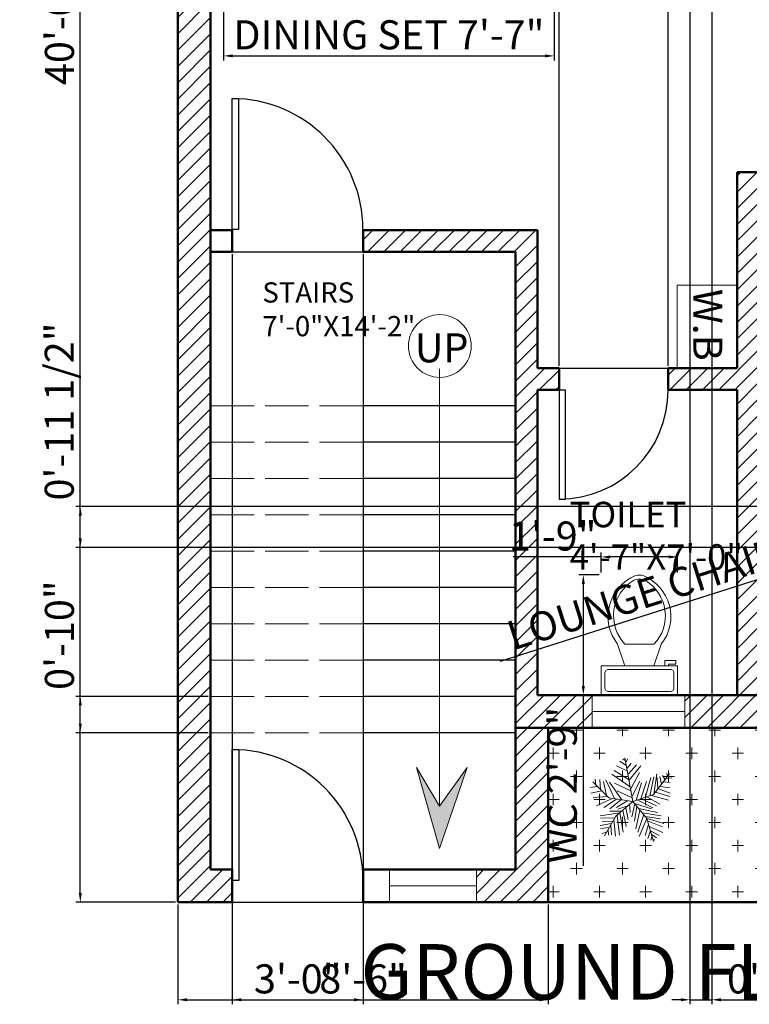
# Model space of a CAD drawing. Units: inches. Extents: x 1188 to 1681, y 1982 to 2608.
# Tile 1 of 4: x 1188 to 1389, y 1988 to 2259. Entities that reach past the tile are written whole.
import ezdxf

# ---------------------------------------------------------------- set-up
doc = ezdxf.new("R2010")
doc.units = ezdxf.units.IN
doc.linetypes.add('ACAD_ISO02W100', pattern=[15, 12, -3])
for name, color, linetype, lineweight in [('A-ANNO-DIMS', 2, 'Continuous', 18), ('A-ANNO-SYMB', 7, 'Continuous', 18), ('A-ANNO-TEXT', 7, 'Continuous', 25), ('A-AREA-IDEN', 7, 'Continuous', 18), ('A-DOOR', 4, 'Continuous', 25), ('A-FLOR-FIXT', 9, 'Continuous', 18), ('A-FLOR-STRS', 7, 'Continuous', 25), ('A-FLOR-STRS-OVHD', 8, 'ACAD_ISO02W100', 18), ('A-GLAZ', 4, 'Continuous', 20), ('A-WALL', 7, 'Continuous', 50), ('A-WALL-PATT', 8, 'Continuous', 13)]:
    doc.layers.add(name, color=color, linetype=linetype, lineweight=lineweight)
doc.layers.add('L-PLNT', color=116, linetype='Continuous', lineweight=18, true_color=0x136734)
doc.layers.add('L-PLNT-PATT', color=116, linetype='Continuous', lineweight=13, true_color=0x136734)
doc.styles.get("Standard").update_dxf_attribs({"font": 'arial.ttf'})
doc.dimstyles.new('ISO-25', dxfattribs={"dimtxt": 8, "dimasz": 2.5, "dimexe": 1.25, "dimexo": 0.625, "dimtad": 1, "dimdec": 1, "dimlunit": 4, "dimtxsty": 'Standard', "dimcen": 2.5, "dimadec": 0, "dimazin": 0, "dimtfac": 1, "dimtdec": 1, "dimtmove": 0, "dimatfit": 3, "dimfxl": 1, "dimarcsym": 0})

# ---------------------------------------------------------------- blocks, each defined once
blk = doc.blocks.new('*U2')
for p, q in [((0, 0), (0, -6)), ((36, 0), (36, -6))]:
    blk.add_line(p, q)
blk.add_lwpolyline([(0, 0), (0, 36), (1.75, 36), (1.75, 0)], close=True)
blk.add_arc((0, 0), 36, 0, 90)
blk = doc.blocks.new('*U3')
for p, q in [((0, 0), (0, 6)), ((30, 0), (30, 6))]:
    blk.add_line(p, q)
blk.add_lwpolyline([(0, 0), (0, -30), (1.75, -30), (1.75, 0)], close=True)
blk.add_arc((0, 0), 30, 270, 0)
blk = doc.blocks.new('Toilet - top')
for p, q in [((9.5, -6), (9.5, -2)), ((-8, -8.5), (-8, -8)), ((-7, -8), (-7, -9.5)), ((-4, -8), (-6, -14)), ((4, -8), (6, -14)), ((-10, -8.5), (-8, -8.5)), ((-10, -9.5), (-10, -8.5)), ((-7, -9.5), (-10, -9.5)), ((4, -14), (-4, -14))]:
    blk.add_line(p, q)
blk.add_lwpolyline([(10.5, -8), (10.5, 0), (-10.5, 0), (-10.5, -8)], close=True)
for points in [[(-9.5, -2), (-9.5, -6)], [(8.5, -1), (-8.5, -1)], [(-8.5, -7), (8.5, -7)]]:
    blk.add_lwpolyline(points)
for centre, radius, start, end in [((-8.62, -1.88), 0.884, 81.8699, 188.1301), ((8.62, -1.88), 0.884, 351.8699, 98.1301), ((-8.62, -6.12), 0.884, 171.8699, 278.1301), ((8.62, -6.12), 0.884, 261.8699, 8.1301), ((3.52, -21.58), 12.17, 141.4691, 247.9714), ((4.2, -21.82), 11.33, 136.3677, 238.9468), ((-3.52, -21.58), 12.17, 292.0284, 38.5307), ((-4.2, -21.82), 11.33, 301.053, 43.6321), ((0, -27.88), 4, 245.7318, 294.2682), ((0, -29), 4, 254.8605, 285.1395)]:
    blk.add_arc(centre, radius, start, end)
blk = doc.blocks.new('*U12')
for p, q in [((-8.737, 47.138), (-17.069, 52.711)), ((-10.186, 53.64), (-13.084, 55.962)), ((0, 0), (-10.5, 57)), ((-9.099, 51.782), (-6.563, 55.962)), ((-5.114, 28.097), (-24.676, 40.636)), ((-7.288, 39.707), (-21.778, 46.673)), ((-7.65, 43.423), (-2.578, 49.46)), ((-5.839, 35.992), (4.667, 48.067)), ((-5.114, 27.632), (10.463, 46.673)), ((-48.585, 21.131), (-49.309, 29.026)), ((-43.513, 28.561), (-42.427, 15.558)), ((-38.442, 26.239), (-34.819, 7.663)), ((-35.544, 28.097), (-24.314, 3.947)), ((-3.665, 19.273), (-27.574, 35.527)), ((-2.941, 16.486), (8.652, 37.85)), ((-1.129, 6.734), (9.014, 26.704)), ((10.101, 3.483), (17.708, 26.239)), ((16.259, 5.805), (23.142, 31.348)), ((22.055, 7.198), (27.489, 32.277)), ((27, 9), (48, 36)), ((27.127, 9.056), (31.112, 35.992)), ((31.836, 30.883), (32.561, 16.486)), ((35.096, 32.741), (37.27, 22.524)), ((38.719, 34.134), (41.979, 28.561)), ((43.791, 29.954), (51.036, 30.883)), ((44.153, 36.456), (45.239, 32.741)), ((-47.498, 19.737), (-55.83, 18.344)), ((-40.615, 13.7), (-55.105, 10.913)), ((-31.5, 4.5), (-52.5, 25.5)), ((-14.533, 2.09), (-30.834, 25.31)), ((-24.314, 23.917), (-2.941, 13.7)), ((-20.691, 13.7), (-1.129, 4.876)), ((3.942, 1.625), (11.187, 24.381)), ((33.285, 16.486), (48.862, 10.913)), ((36.183, 19.737), (48.137, 17.88)), ((40.53, 25.775), (48.862, 24.846)), ((-33.37, 6.269), (-52.207, 5.34)), ((-28.299, 3.483), (-47.86, -5.805)), ((-21.416, 3.018), (-38.079, -8.128)), ((0, 0), (-31.5, 4.5)), ((-15.982, 2.09), (-30.11, -9.521)), ((0, 0), (-22.5, -19.5)), ((-6.563, 1.161), (-21.416, -8.128)), ((0, 0), (27, 9)), ((0, 0), (18, -22.5)), ((6.478, 1.625), (26.04, -8.592)), ((11.187, 3.483), (30.749, -5.805)), ((18.07, 5.805), (35.096, -3.483)), ((24.229, 7.663), (46.688, 1.625)), ((29.662, 12.307), (48.137, 6.269)), ((-15.257, -12.772), (-30.11, -12.772)), ((-6.563, -5.805), (-19.967, -9.985)), ((-13.446, -11.378), (-8.737, -32.741)), ((-9.461, -8.592), (-6.201, -23.453)), ((-4.752, -3.483), (-3.665, -14.629)), ((2.493, -3.019), (-1.491, -20.202)), ((1.769, -2.555), (24.229, -9.521)), ((5.029, -6.27), (2.131, -25.775)), ((9.014, -11.378), (3.58, -35.992)), ((7.565, -9.056), (32.198, -14.629)), ((-17.431, -15.094), (-42.789, -18.809)), ((-24.314, -21.596), (-42.427, -22.06)), ((-26.849, -26.24), (-40.253, -25.775)), ((-22.5, -19.5), (-37.5, -45)), ((-25.038, -23.918), (-22.865, -45.281)), ((-20.691, -18.345), (-17.793, -44.352)), ((-17.069, -15.094), (-12.721, -40.172)), ((14.085, -16.951), (6.478, -40.172)), ((18.07, -22.524), (8.289, -45.745)), ((12.274, -15.094), (36.907, -18.809)), ((16.259, -19.738), (36.183, -22.989)), ((18, -22.5), (27, -52.5)), ((18.433, -22.524), (40.53, -29.026)), ((19.157, -25.311), (38.719, -33.206)), ((-28.299, -29.026), (-42.789, -31.348)), ((-30.834, -34.135), (-42.427, -35.528)), ((-32.646, -36.921), (-31.921, -44.352)), ((-29.023, -30.884), (-27.936, -43.887)), ((20.244, -30.419), (15.897, -44.816)), ((22.78, -37.85), (19.519, -48.532)), ((21.331, -32.741), (39.081, -40.636)), ((22.78, -38.314), (34.372, -44.816)), ((-34.457, -39.708), (-40.978, -42.494)), ((24.591, -45.745), (23.142, -50.854)), ((24.591, -43.423), (30.749, -47.603)), ((26.764, -49.925), (28.213, -50.854))]:
    blk.add_line(p, q)
blk = doc.blocks.new('*D30')
at = {"layer": 'A-ANNO-DIMS', "color": 0, "lineweight": -2, "transparency": 16777216}
for p, q in [((1498.32, 2135.79), (1496.92, 2140.18)), ((1494.92, 2138.23), (1474.36, 2131.69)), ((1471.98, 2130.93), (1320.5, 2082.67)), ((1473, 2127.73), (1471.6, 2132.12))]:
    blk.add_line(p, q, dxfattribs=at)
at = {"layer": 'A-ANNO-DIMS', "color": 0, "transparency": 16777216}
for points in [[(1494.79, 2138.63), (1495.04, 2137.84), (1497.3, 2138.99)], [(1474.24, 2132.08), (1474.49, 2131.29), (1471.98, 2130.93)]]:
    blk.add_solid(points, dxfattribs=at)
at = {"layer": 'Defpoints', "color": 0, "transparency": 16777216}
for p in [(1498.51, 2135.2), (1471.98, 2130.93), (1473.19, 2127.13)]:
    blk.add_point(p, dxfattribs=at)
at = {"layer": 'A-ANNO-DIMS', "color": 0, "transparency": 16777216, "insert": (1393.6, 2110.96), "char_height": 8, "attachment_point": 5, "rotation": 17.6695}
blk.add_mtext('LOUNGE CHAIR 2\'-2 1/2" TYP.', dxfattribs=at)
blk = doc.blocks.new('*D32')
at = {"layer": 'A-ANNO-DIMS', "color": 0, "lineweight": -2, "transparency": 16777216}
for p, q in [((1419.52, 2095.98), (1419.52, 2243.74)), ((1418.76, 2095.98), (1420.77, 2095.98)), ((1419.52, 2089.2), (1419.52, 2093.48)), ((1418.76, 2086.7), (1420.77, 2086.7))]:
    blk.add_line(p, q, dxfattribs=at)
at = {"layer": 'A-ANNO-DIMS', "color": 0, "transparency": 16777216}
for points in [[(1419.11, 2093.48), (1419.94, 2093.48), (1419.52, 2095.98)], [(1419.11, 2089.2), (1419.94, 2089.2), (1419.52, 2086.7)]]:
    blk.add_solid(points, dxfattribs=at)
at = {"layer": 'Defpoints', "color": 0, "transparency": 16777216}
for p in [(1418.13, 2095.98), (1419.52, 2095.98), (1418.13, 2086.7)]:
    blk.add_point(p, dxfattribs=at)
at = {"layer": 'A-ANNO-DIMS', "color": 0, "transparency": 16777216, "insert": (1414.76, 2171.11), "char_height": 8, "attachment_point": 5, "rotation": 90}
blk.add_mtext('RADIAL LAMP 0\'-9 1/2" TYP.', dxfattribs=at)
blk = doc.blocks.new('*D38')
at = {"layer": 'A-ANNO-DIMS', "color": 0, "lineweight": -2, "transparency": 16777216}
for p, q in [((1244.32, 2262.4), (1244.32, 2248.12)), ((1335.32, 2262.4), (1335.32, 2248.12)), ((1246.82, 2249.37), (1332.82, 2249.37))]:
    blk.add_line(p, q, dxfattribs=at)
at = {"layer": 'A-ANNO-DIMS', "color": 0, "transparency": 16777216}
for points in [[(1246.82, 2249.79), (1246.82, 2248.96), (1244.32, 2249.37)], [(1332.82, 2249.79), (1332.82, 2248.96), (1335.32, 2249.37)]]:
    blk.add_solid(points, dxfattribs=at)
at = {"layer": 'Defpoints', "color": 0, "transparency": 16777216}
for p in [(1244.32, 2263.02), (1335.32, 2263.02), (1335.32, 2249.37)]:
    blk.add_point(p, dxfattribs=at)
at = {"layer": 'A-ANNO-DIMS', "color": 0, "transparency": 16777216, "insert": (1289.82, 2254.14), "char_height": 8, "attachment_point": 5}
blk.add_mtext('DINING SET 7\'-7"', dxfattribs=at)
blk = doc.blocks.new('*D42')
at = {"layer": 'A-ANNO-DIMS', "color": 0, "lineweight": -2, "transparency": 16777216}
for p, q in [((1347.68, 2106.5), (1342.1, 2106.5)), ((1343.35, 2104), (1343.35, 2075.96)), ((1347.68, 2073.46), (1342.1, 2073.46)), ((1343.35, 2073.46), (1343.35, 2026.39))]:
    blk.add_line(p, q, dxfattribs=at)
at = {"layer": 'A-ANNO-DIMS', "color": 0, "transparency": 16777216}
for points in [[(1342.93, 2104), (1343.77, 2104), (1343.35, 2106.5)], [(1342.93, 2075.96), (1343.77, 2075.96), (1343.35, 2073.46)]]:
    blk.add_solid(points, dxfattribs=at)
at = {"layer": 'Defpoints', "color": 0, "transparency": 16777216}
for p in [(1348.31, 2106.5), (1343.35, 2073.46), (1348.31, 2073.46)]:
    blk.add_point(p, dxfattribs=at)
at = {"layer": 'A-ANNO-DIMS', "color": 0, "transparency": 16777216, "insert": (1338.59, 2048.67), "char_height": 8, "attachment_point": 5, "rotation": 90}
blk.add_mtext('WC 2\'-9"', dxfattribs=at)
blk = doc.blocks.new('*D43')
at = {"layer": 'A-ANNO-DIMS', "color": 0, "lineweight": -2, "transparency": 16777216}
for p, q in [((1348.31, 2111.46), (1324.04, 2111.46)), ((1348.31, 2107.13), (1348.31, 2112.71)), ((1366.81, 2111.46), (1350.81, 2111.46)), ((1369.31, 2107.13), (1369.31, 2112.71))]:
    blk.add_line(p, q, dxfattribs=at)
at = {"layer": 'A-ANNO-DIMS', "color": 0, "transparency": 16777216}
for points in [[(1350.81, 2111.88), (1350.81, 2111.04), (1348.31, 2111.46)], [(1366.81, 2111.88), (1366.81, 2111.04), (1369.31, 2111.46)]]:
    blk.add_solid(points, dxfattribs=at)
at = {"layer": 'Defpoints', "color": 0, "transparency": 16777216}
for p in [(1348.31, 2111.46), (1348.31, 2106.5), (1369.31, 2106.5)]:
    blk.add_point(p, dxfattribs=at)
at = {"layer": 'A-ANNO-DIMS', "color": 0, "transparency": 16777216, "insert": (1334.93, 2116.17), "char_height": 8, "attachment_point": 5}
blk.add_mtext('1\'-9"', dxfattribs=at)
blk = doc.blocks.new('*D44')
at = {"layer": 'A-ANNO-DIMS', "color": 0, "lineweight": -2, "transparency": 16777216}
for p, q in [((1231.09, 2496.41), (1203.62, 2496.41)), ((1204.87, 2018.91), (1204.87, 2493.91)), ((1231.09, 2016.41), (1203.62, 2016.41))]:
    blk.add_line(p, q, dxfattribs=at)
at = {"layer": 'A-ANNO-DIMS', "color": 0, "transparency": 16777216}
for points in [[(1204.45, 2493.91), (1205.28, 2493.91), (1204.87, 2496.41)], [(1204.45, 2018.91), (1205.28, 2018.91), (1204.87, 2016.41)]]:
    blk.add_solid(points, dxfattribs=at)
at = {"layer": 'Defpoints', "color": 0, "transparency": 16777216}
for p in [(1204.87, 2496.41), (1231.72, 2496.41), (1231.72, 2016.41)]:
    blk.add_point(p, dxfattribs=at)
at = {"layer": 'A-ANNO-DIMS', "color": 0, "transparency": 16777216, "insert": (1200.16, 2256.41), "char_height": 8, "attachment_point": 5, "rotation": 90}
blk.add_mtext('40\'-0"', dxfattribs=at)
blk = doc.blocks.new('*D45')
at = {"layer": 'A-ANNO-DIMS', "color": 0, "lineweight": -2, "transparency": 16777216}
for p, q in [((1246.72, 2015.79), (1246.72, 1988.31)), ((1282.72, 2015.79), (1282.72, 1988.31)), ((1249.22, 1989.56), (1280.22, 1989.56))]:
    blk.add_line(p, q, dxfattribs=at)
at = {"layer": 'A-ANNO-DIMS', "color": 0, "transparency": 16777216}
for points in [[(1249.22, 1989.98), (1249.22, 1989.15), (1246.72, 1989.56)], [(1280.22, 1989.98), (1280.22, 1989.15), (1282.72, 1989.56)]]:
    blk.add_solid(points, dxfattribs=at)
at = {"layer": 'Defpoints', "color": 0, "transparency": 16777216}
for p in [(1246.72, 2016.41), (1282.72, 2016.41), (1282.72, 1989.56)]:
    blk.add_point(p, dxfattribs=at)
at = {"layer": 'A-ANNO-DIMS', "color": 0, "transparency": 16777216, "insert": (1264.72, 1994.28), "char_height": 8, "attachment_point": 5}
blk.add_mtext('3\'-0"', dxfattribs=at)
blk = doc.blocks.new('*D46')
at = {"layer": 'A-ANNO-DIMS', "color": 0, "lineweight": -2, "transparency": 16777216}
for p, q in [((1204.87, 2073.07), (1204.87, 2104.3)), ((1240.09, 2073.07), (1203.62, 2073.07)), ((1204.87, 2065.57), (1204.87, 2070.57)), ((1240.09, 2063.07), (1203.62, 2063.07))]:
    blk.add_line(p, q, dxfattribs=at)
at = {"layer": 'A-ANNO-DIMS', "color": 0, "transparency": 16777216}
for points in [[(1204.45, 2070.57), (1205.28, 2070.57), (1204.87, 2073.07)], [(1204.45, 2065.57), (1205.28, 2065.57), (1204.87, 2063.07)]]:
    blk.add_solid(points, dxfattribs=at)
at = {"layer": 'Defpoints', "color": 0, "transparency": 16777216}
for p in [(1204.87, 2073.07), (1240.72, 2073.07), (1240.72, 2063.07)]:
    blk.add_point(p, dxfattribs=at)
at = {"layer": 'A-ANNO-DIMS', "color": 0, "transparency": 16777216, "insert": (1200.16, 2089.93), "char_height": 8, "attachment_point": 5, "rotation": 90}
blk.add_mtext('0\'-10"', dxfattribs=at)
blk = doc.blocks.new('*D47')
at = {"layer": 'A-ANNO-DIMS', "color": 0, "lineweight": -2, "transparency": 16777216}
for p, q in [((1336.72, 2164.04), (1336.72, 2524.51)), ((1339.22, 2523.26), (1364.22, 2523.26)), ((1366.72, 2164.04), (1366.72, 2524.51))]:
    blk.add_line(p, q, dxfattribs=at)
at = {"layer": 'A-ANNO-DIMS', "color": 0, "transparency": 16777216}
for points in [[(1339.22, 2523.68), (1339.22, 2522.85), (1336.72, 2523.26)], [(1364.22, 2523.68), (1364.22, 2522.85), (1366.72, 2523.26)]]:
    blk.add_solid(points, dxfattribs=at)
at = {"layer": 'Defpoints', "color": 0, "transparency": 16777216}
for p in [(1366.72, 2523.26), (1336.72, 2163.41), (1366.72, 2163.41)]:
    blk.add_point(p, dxfattribs=at)
at = {"layer": 'A-ANNO-DIMS', "color": 0, "transparency": 16777216, "insert": (1351.72, 2527.97), "char_height": 8, "attachment_point": 5}
blk.add_mtext('2\'-6"', dxfattribs=at)
blk = doc.blocks.new('*D49')
at = {"layer": 'A-ANNO-DIMS', "color": 0, "lineweight": -2, "transparency": 16777216}
for p, q in [((1231.72, 2015.79), (1231.72, 1988.31)), ((1333.72, 2015.79), (1333.72, 1988.31)), ((1234.22, 1989.56), (1331.22, 1989.56))]:
    blk.add_line(p, q, dxfattribs=at)
at = {"layer": 'A-ANNO-DIMS', "color": 0, "transparency": 16777216}
for points in [[(1234.22, 1989.98), (1234.22, 1989.15), (1231.72, 1989.56)], [(1331.22, 1989.98), (1331.22, 1989.15), (1333.72, 1989.56)]]:
    blk.add_solid(points, dxfattribs=at)
at = {"layer": 'Defpoints', "color": 0, "transparency": 16777216}
for p in [(1231.72, 2016.41), (1333.72, 2016.41), (1333.72, 1989.56)]:
    blk.add_point(p, dxfattribs=at)
at = {"layer": 'A-ANNO-DIMS', "color": 0, "transparency": 16777216, "insert": (1282.72, 1994.27), "char_height": 8, "attachment_point": 5}
blk.add_mtext('8\'-6"', dxfattribs=at)
blk = doc.blocks.new('*D50')
at = {"layer": 'A-ANNO-DIMS', "color": 0, "lineweight": -2, "transparency": 16777216}
for p, q in [((1372.72, 2342.79), (1372.72, 1988.31)), ((1378.72, 2336.79), (1378.72, 1988.31)), ((1370.22, 1989.56), (1367.72, 1989.56)), ((1372.72, 1989.56), (1378.72, 1989.56)), ((1381.22, 1989.56), (1406.23, 1989.56))]:
    blk.add_line(p, q, dxfattribs=at)
at = {"layer": 'A-ANNO-DIMS', "color": 0, "transparency": 16777216}
for points in [[(1370.22, 1989.98), (1370.22, 1989.15), (1372.72, 1989.56)], [(1381.22, 1989.98), (1381.22, 1989.15), (1378.72, 1989.56)]]:
    blk.add_solid(points, dxfattribs=at)
at = {"layer": 'Defpoints', "color": 0, "transparency": 16777216}
for p in [(1372.72, 2343.41), (1378.72, 2337.41), (1378.72, 1989.56)]:
    blk.add_point(p, dxfattribs=at)
at = {"layer": 'A-ANNO-DIMS', "color": 0, "transparency": 16777216, "insert": (1394.97, 1994.27), "char_height": 8, "attachment_point": 5}
blk.add_mtext('0\'-6"', dxfattribs=at)
blk = doc.blocks.new('*D56')
at = {"layer": 'A-ANNO-DIMS', "color": 0, "lineweight": -2, "transparency": 16777216}
for p, q in [((1246.72, 2194.79), (1246.72, 1988.31)), ((1282.72, 2194.79), (1282.72, 1988.31)), ((1249.22, 1989.56), (1280.22, 1989.56))]:
    blk.add_line(p, q, dxfattribs=at)
at = {"layer": 'A-ANNO-DIMS', "color": 0, "transparency": 16777216}
for points in [[(1249.22, 1989.98), (1249.22, 1989.15), (1246.72, 1989.56)], [(1280.22, 1989.98), (1280.22, 1989.15), (1282.72, 1989.56)]]:
    blk.add_solid(points, dxfattribs=at)
at = {"layer": 'Defpoints', "color": 0, "transparency": 16777216}
for p in [(1246.72, 2195.41), (1282.72, 2195.41), (1282.72, 1989.56)]:
    blk.add_point(p, dxfattribs=at)
at = {"layer": 'A-ANNO-DIMS', "color": 0, "transparency": 16777216, "insert": (1264.72, 1994.28), "char_height": 8, "attachment_point": 5}
blk.add_mtext('3\'-0"', dxfattribs=at)
blk = doc.blocks.new('*D58')
at = {"layer": 'A-ANNO-DIMS', "color": 0, "lineweight": -2, "transparency": 16777216}
for p, q in [((1204.87, 2125.31), (1204.87, 2175.18)), ((1439.4, 2125.31), (1203.62, 2125.31)), ((1204.87, 2116.54), (1204.87, 2122.81)), ((1439.4, 2114.04), (1203.62, 2114.04))]:
    blk.add_line(p, q, dxfattribs=at)
at = {"layer": 'A-ANNO-DIMS', "color": 0, "transparency": 16777216}
for points in [[(1204.45, 2122.81), (1205.28, 2122.81), (1204.87, 2125.31)], [(1204.45, 2116.54), (1205.28, 2116.54), (1204.87, 2114.04)]]:
    blk.add_solid(points, dxfattribs=at)
at = {"layer": 'Defpoints', "color": 0, "transparency": 16777216}
for p in [(1204.87, 2125.31), (1440.02, 2125.31), (1440.02, 2114.04)]:
    blk.add_point(p, dxfattribs=at)
at = {"layer": 'A-ANNO-DIMS', "color": 0, "transparency": 16777216, "insert": (1200.11, 2151.49), "char_height": 8, "attachment_point": 5, "rotation": 90}
blk.add_mtext('0\'-11 1/2"', dxfattribs=at)

msp = doc.modelspace()

# ---------------------------------------------------------------- hatches: boundary and pattern name
at = {"layer": 'A-ANNO-SYMB', "transparency": 33554564}
h = msp.add_hatch(color=256, dxfattribs=at)
h.dxf.hatch_style = 1
h.paths.add_polyline_path([(1311.34, 2053.46), (1303.72, 2042.82), (1297.4, 2053.46), (1303.72, 2031.22)])
at = {"layer": 'A-WALL-PATT', "transparency": 33554559}
h = msp.add_hatch(dxfattribs=at)
h.set_pattern_fill('ANSI31', color=256)
h.paths.add_polyline_path([(1390.99, 2496.41), (1231.72, 2496.41), (1231.72, 2452.82), (1240.72, 2452.82), (1240.72, 2487.41), (1390.99, 2487.41)])
h.paths.add_polyline_path([(1469.3, 2496.41), (1426.99, 2496.41), (1426.99, 2491.91), (1426.99, 2487.41), (1469.3, 2487.41)])
h.paths.add_polyline_path([(1378.72, 2487.41), (1372.72, 2487.41), (1372.72, 2404.84), (1372.72, 2343.41), (1367.48, 2343.41), (1367.48, 2337.41), (1378.72, 2337.41), (1378.72, 2391.41), (1387.67, 2391.41), (1387.67, 2397.41), (1378.72, 2397.41)])
h.paths.add_polyline_path([(1438.72, 2487.41), (1432.72, 2487.41), (1432.72, 2397.41), (1420.72, 2397.41), (1420.72, 2391.41), (1432.72, 2391.41), (1432.72, 2385.41), (1438.72, 2385.41)])
h.paths.add_polyline_path([(1240.72, 2392.82), (1236.22, 2392.82), (1231.72, 2392.82), (1231.72, 2323.77), (1240.72, 2323.77)])
h.paths.add_polyline_path([(1330.72, 2343.41), (1240.72, 2343.41), (1240.72, 2337.41), (1330.72, 2337.41)])
h.paths.add_polyline_path([(1558.72, 2343.41), (1438.72, 2343.41), (1438.72, 2349.29), (1438.64, 2349.29), (1432.72, 2349.29), (1432.72, 2259.41), (1438.72, 2259.41), (1438.72, 2337.41), (1558.72, 2337.41)])
h.paths.add_polyline_path([(1567.72, 2396.81), (1558.72, 2396.81), (1558.72, 2317.68), (1563.22, 2317.68), (1567.72, 2317.68)])
h.paths.add_polyline_path([(1567.72, 2496.41), (1529.3, 2496.41), (1529.3, 2491.91), (1529.3, 2487.41), (1558.72, 2487.41), (1558.72, 2461.81), (1567.72, 2461.81)])
h.paths.add_polyline_path([(1240.72, 2195.41), (1240.72, 2201.41), (1240.72, 2263.77), (1231.72, 2263.77), (1231.72, 2016.41), (1246.72, 2016.41), (1246.72, 2022.41), (1246.72, 2025.41), (1240.72, 2025.41)])
h.paths.add_polyline_path([(1391.72, 2211.41), (1397.72, 2211.41), (1397.72, 2217.41), (1385.72, 2217.41), (1385.72, 2163.41), (1366.72, 2163.41), (1366.72, 2157.41), (1385.72, 2157.41), (1385.72, 2073.41), (1391.72, 2073.41)])
h.paths.add_polyline_path([(1330.72, 2201.41), (1282.72, 2201.41), (1282.72, 2195.41), (1324.72, 2195.41), (1324.72, 2064.41), (1345.75, 2064.41), (1345.75, 2073.41), (1330.72, 2073.41), (1330.72, 2157.41), (1336.72, 2157.41), (1336.72, 2163.41), (1330.72, 2163.41)])
h.paths.add_polyline_path([(1558.72, 2217.41), (1438.72, 2217.41), (1438.72, 2223.26), (1432.72, 2223.26), (1432.72, 2217.41), (1427.72, 2217.41), (1427.72, 2211.41), (1432.72, 2211.41), (1558.72, 2211.41)])
h.paths.add_polyline_path([(1567.72, 2269.68), (1558.72, 2269.68), (1558.72, 2182.72), (1563.22, 2182.72), (1567.72, 2182.72)])
h.paths.add_polyline_path([(1567.72, 2134.72), (1558.72, 2134.72), (1558.72, 2073.41), (1497.85, 2073.41), (1497.85, 2068.91), (1497.85, 2064.41), (1567.72, 2064.41)])
h.paths.add_polyline_path([(1449.85, 2073.41), (1371.31, 2073.41), (1371.31, 2068.91), (1371.31, 2064.41), (1449.85, 2064.41)])
h.paths.add_polyline_path([(1333.72, 2064.41), (1324.72, 2064.41), (1324.72, 2025.41), (1313.9, 2025.41), (1313.9, 2016.41), (1333.72, 2016.41)])
at = {"layer": 'L-PLNT-PATT', "transparency": 33554679}
h = msp.add_hatch(dxfattribs=at)
h.set_pattern_fill('CROSS', color=256)
h.paths.add_polyline_path([(1567.72, 2064.41), (1333.72, 2064.41), (1333.72, 2016.41), (1567.72, 2016.41)])

# ---------------------------------------------------------------- linework, layer by layer
at = {"layer": 'A-ANNO-SYMB'}
for p, q in [((1303.72, 2163.2), (1303.72, 2042.82)), ((1303.72, 2042.82), (1297.4, 2053.46)), ((1297.4, 2053.46), (1303.72, 2031.22)), ((1303.72, 2031.22), (1311.34, 2053.46)), ((1311.34, 2053.46), (1303.72, 2042.82))]:
    msp.add_line(p, q, dxfattribs=at)
msp.add_circle((1303.84, 2169.52), 8.64, dxfattribs=at)
at = {"layer": 'A-DOOR'}
for p, q in [((1246.72, 2195.41), (1282.72, 2195.41)), ((1336.72, 2163.41), (1366.72, 2163.41)), ((1246.72, 2016.41), (1282.72, 2016.41))]:
    msp.add_line(p, q, dxfattribs=at)
at = {"layer": 'A-FLOR-FIXT'}
for p, q in [((1385.72, 2186.25), (1369.22, 2186.25)), ((1369.22, 2186.25), (1369.22, 2163.41)), ((1385.72, 2186.25), (1385.72, 2186.25))]:
    msp.add_line(p, q, dxfattribs=at)
at = {"layer": 'A-FLOR-STRS'}
for p, q in [((1324.72, 2153.07), (1282.72, 2153.07)), ((1282.72, 2153.07), (1282.72, 2063.07)), ((1324.72, 2143.07), (1282.72, 2143.07)), ((1324.72, 2133.07), (1282.72, 2133.07)), ((1324.72, 2123.07), (1282.72, 2123.07)), ((1324.72, 2113.07), (1282.72, 2113.07)), ((1324.72, 2103.07), (1282.72, 2103.07)), ((1324.72, 2093.07), (1282.72, 2093.07)), ((1324.72, 2083.07), (1282.72, 2083.07)), ((1324.72, 2073.07), (1282.72, 2073.07)), ((1324.72, 2063.07), (1282.72, 2063.07))]:
    msp.add_line(p, q, dxfattribs=at)
at = {"layer": 'A-FLOR-STRS-OVHD'}
for p, q in [((1282.72, 2153.07), (1240.72, 2153.07)), ((1282.72, 2143.07), (1240.72, 2143.07)), ((1282.72, 2133.07), (1240.72, 2133.07)), ((1282.72, 2123.07), (1240.72, 2123.07)), ((1282.72, 2113.07), (1240.72, 2113.07)), ((1282.72, 2103.07), (1240.72, 2103.07)), ((1282.72, 2093.07), (1240.72, 2093.07)), ((1282.72, 2083.07), (1240.72, 2083.07)), ((1282.72, 2073.07), (1240.72, 2073.07)), ((1282.72, 2063.07), (1240.72, 2063.07))]:
    msp.add_line(p, q, dxfattribs=at)
at = {"layer": 'A-GLAZ'}
for p, q in [((1345.75, 2073.41), (1345.75, 2064.41)), ((1371.31, 2064.41), (1371.31, 2073.41)), ((1371.31, 2073.41), (1371.31, 2068.91)), ((1371.31, 2068.91), (1345.75, 2068.91)), ((1345.75, 2064.41), (1371.31, 2064.41)), ((1289.97, 2025.41), (1289.97, 2016.41)), ((1313.9, 2020.91), (1313.9, 2025.41)), ((1313.9, 2025.41), (1313.9, 2016.41)), ((1289.97, 2016.41), (1289.97, 2020.91)), ((1289.97, 2020.91), (1313.9, 2020.91))]:
    msp.add_line(p, q, dxfattribs=at)
at = {"layer": 'A-WALL'}
for p, q in [((1231.72, 2496.41), (1231.72, 2016.41)), ((1240.72, 2487.41), (1240.72, 2201.41)), ((1385.72, 2217.41), (1385.72, 2163.41)), ((1385.72, 2217.41), (1397.72, 2217.41)), ((1240.72, 2201.41), (1246.72, 2201.41)), ((1240.72, 2201.41), (1240.72, 2195.41)), ((1246.72, 2201.41), (1246.72, 2195.41)), ((1282.72, 2201.41), (1282.72, 2195.41)), ((1282.72, 2201.41), (1330.72, 2201.41)), ((1330.72, 2201.41), (1330.72, 2163.41)), ((1240.72, 2195.41), (1246.72, 2195.41)), ((1240.72, 2195.41), (1240.72, 2025.41)), ((1282.72, 2195.41), (1324.72, 2195.41)), ((1324.72, 2195.41), (1324.72, 2025.41)), ((1330.72, 2163.41), (1336.72, 2163.41)), ((1336.72, 2163.41), (1336.72, 2157.41)), ((1366.72, 2163.41), (1366.72, 2157.41)), ((1366.72, 2163.41), (1385.72, 2163.41)), ((1330.72, 2157.41), (1336.72, 2157.41)), ((1330.72, 2157.41), (1330.72, 2073.41)), ((1366.72, 2157.41), (1385.72, 2157.41)), ((1385.72, 2157.41), (1385.72, 2073.41)), ((1330.72, 2073.41), (1558.72, 2073.41)), ((1324.72, 2064.41), (1567.72, 2064.41)), ((1333.72, 2064.41), (1333.72, 2016.41)), ((1240.72, 2025.41), (1246.72, 2025.41)), ((1246.72, 2025.41), (1246.72, 2016.41)), ((1282.72, 2025.41), (1282.72, 2016.41)), ((1282.72, 2025.41), (1324.72, 2025.41)), ((1231.72, 2016.41), (1246.72, 2016.41)), ((1282.72, 2016.41), (1567.72, 2016.41))]:
    msp.add_line(p, q, dxfattribs=at)

# ---------------------------------------------------------------- block references
at = {"layer": 'A-DOOR'}
for name, p in [('*U2', (1246.67, 2201.63)), ('*U3', (1336.72, 2157.36)), ('*U2', (1246.72, 2022.41))]:
    msp.add_blockref(name, p, dxfattribs=at)
at = {"layer": 'A-FLOR-FIXT', "rotation": 180}
msp.add_blockref('Toilet - top', (1358.81, 2073.46), dxfattribs=at)
at = {"layer": 'L-PLNT', "xscale": 0.2102822374520575, "yscale": 0.2102822374520575, "zscale": 0.2102822374520575}
msp.add_blockref('*U12', (1357.03, 2044.16), dxfattribs=at)

# ---------------------------------------------------------------- texts
at = {"layer": 'A-ANNO-TEXT', "insert": (1296.96, 2173.02), "char_height": 8, "attachment_point": 1}
msp.add_mtext('UP', dxfattribs=at)
at = {"layer": 'A-ANNO-TEXT', "insert": (1281.99, 2004.88), "char_height": 15.2538, "attachment_point": 1}
msp.add_mtext_dynamic_manual_height_columns('GROUND FLOOR PLAN', width=268.1014, gutter_width=23.83, heights=[0], dxfattribs=at)
at = {"layer": 'A-AREA-IDEN', "insert": (1254.99, 2187.05), "char_height": 5.5661, "attachment_point": 1}
msp.add_mtext_dynamic_manual_height_columns('STAIRS\\P7\'-0"X14\'-2"', width=1.7394, gutter_width=8.7, heights=[0], dxfattribs=at)
at = {"layer": 'A-AREA-IDEN', "insert": (1381.64, 2185.24), "char_height": 8, "attachment_point": 1, "rotation": 270}
msp.add_mtext('W.B', dxfattribs=at)
at = {"layer": 'A-AREA-IDEN', "insert": (1339.6, 2126.63), "char_height": 7, "attachment_point": 1}
msp.add_mtext('TOILET\\P4\'-7"X7\'-0"', dxfattribs=at)

# ---------------------------------------------------------------- dimensions: what is measured, and where the dimension line sits
at = {"layer": 'A-ANNO-DIMS'}
for base, p1, p2, picture, middle in [((1366.72, 2523.26), (1336.72, 2163.41), (1366.72, 2163.41), '*D47', (1351.72, 2527.97)), ((1378.72, 1989.56), (1372.72, 2343.41), (1378.72, 2337.41), '*D50', (1394.97, 1994.27)), ((1282.72, 1989.56), (1246.72, 2195.41), (1282.72, 2195.41), '*D56', (1264.72, 1994.28)), ((1333.72, 1989.56), (1231.72, 2016.41), (1333.72, 2016.41), '*D49', (1282.72, 1994.27)), ((1282.72, 1989.56), (1246.72, 2016.41), (1282.72, 2016.41), '*D45', (1264.72, 1994.28))]:
    dim = msp.add_linear_dim(base=base, p1=p1, p2=p2, dimstyle='ISO-25', override={"dimdec": 1, "dimlfac": 1, "dimrnd": 0, "dimzin": 1, "dimdsep": 46, "dimlunit": 4, "dimfrac": 2}, dxfattribs=at)
    dim.commit()
    dim.dimension.update_dxf_attribs({"geometry": picture, "text_midpoint": middle})
for base, p1, p2, angle, picture, middle in [((1204.87, 2496.41), (1231.72, 2016.41), (1231.72, 2496.41), 90, '*D44', (1200.16, 2256.41)), ((1204.87, 2125.31), (1440.02, 2114.04), (1440.02, 2125.31), 90, '*D58', (1200.11, 2151.49)), ((1348.31, 2111.46), (1369.31, 2106.5), (1348.31, 2106.5), 180, '*D43', (1334.93, 2116.17)), ((1204.87, 2073.07), (1240.72, 2063.07), (1240.72, 2073.07), 90, '*D46', (1200.16, 2089.93))]:
    dim = msp.add_linear_dim(base=base, p1=p1, p2=p2, angle=angle, dimstyle='ISO-25', override={"dimdec": 1, "dimlfac": 1, "dimrnd": 0, "dimzin": 1, "dimdsep": 46, "dimlunit": 4, "dimfrac": 2}, dxfattribs=at)
    dim.commit()
    dim.dimension.update_dxf_attribs({"geometry": picture, "text_midpoint": middle})
dim = msp.add_linear_dim(base=(1335.32, 2249.37), p1=(1244.32, 2263.02), p2=(1335.32, 2263.02), text='DINING SET <>', dimstyle='ISO-25', override={"dimdec": 1, "dimlfac": 1, "dimrnd": 0, "dimzin": 1, "dimdsep": 46, "dimlunit": 4, "dimfrac": 2}, dxfattribs=at)
dim.commit()
dim.dimension.update_dxf_attribs({"geometry": '*D38', "text_midpoint": (1289.82, 2254.14)})
for base, p1, p2, angle, text, picture, middle in [((1419.52, 2095.98), (1418.13, 2086.7), (1418.13, 2095.98), 90, 'RADIAL LAMP <> TYP.', '*D32', (1414.76, 2171.11)), ((1471.98, 2130.93), (1498.51, 2135.2), (1473.19, 2127.13), 197.6695, 'LOUNGE CHAIR <> TYP.', '*D30', (1393.6, 2110.96)), ((1343.35, 2073.46), (1348.31, 2106.5), (1348.31, 2073.46), 270, 'WC <>', '*D42', (1338.59, 2048.67))]:
    dim = msp.add_linear_dim(base=base, p1=p1, p2=p2, angle=angle, text=text, dimstyle='ISO-25', override={"dimdec": 1, "dimlfac": 1, "dimrnd": 0, "dimzin": 1, "dimdsep": 46, "dimlunit": 4, "dimfrac": 2}, dxfattribs=at)
    dim.commit()
    dim.dimension.update_dxf_attribs({"geometry": picture, "text_midpoint": middle})

doc.saveas('drawing.dxf')
